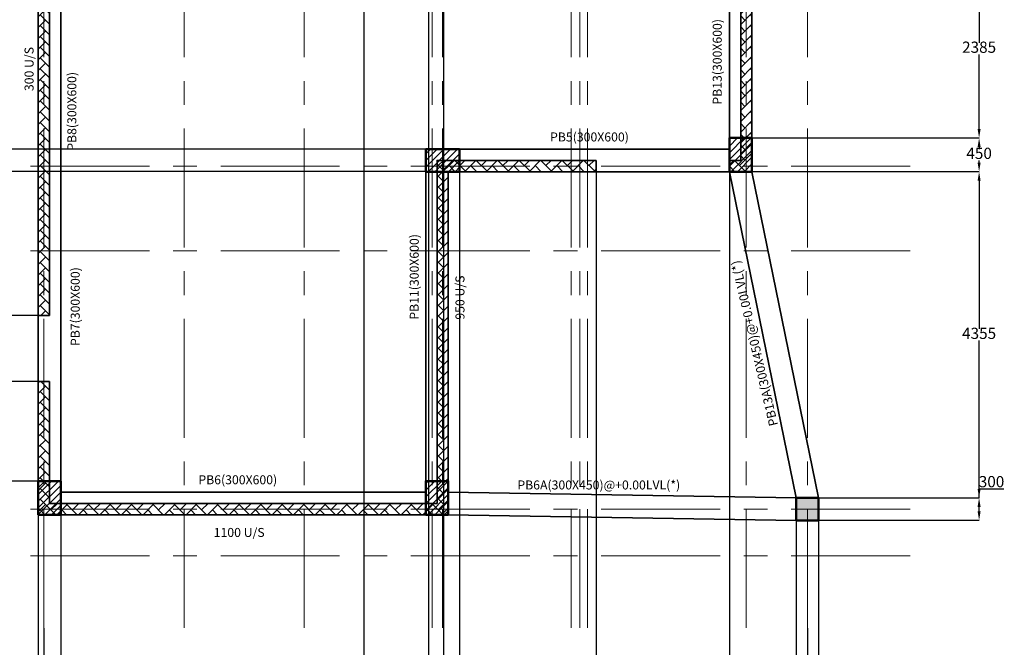
# Model space of a CAD drawing. Units: millimetres. Extents: x -174 to 32373, y 27344 to 53129.
# Tile 4 of 7: x 8204 to 21352, y 36674 to 45053. Entities that reach past the tile are written whole.
import ezdxf

# ---------------------------------------------------------------- set-up
doc = ezdxf.new("R2010")
doc.units = ezdxf.units.MM
doc.header["$LTSCALE"] = 50
doc.linetypes.add('CENTER', pattern=[50.8, 31.75, -6.35, 6.35, -6.35])
for name, color, linetype, lineweight in [('S-ANNO-DIMS', 2, 'Continuous', 18), ('S-ANNO-TEXT', 3, 'Continuous', 18), ('S-BEAM', 7, 'Continuous', 35), ('S-COLS', 1, 'Continuous', 50), ('S-GRID', 8, 'CENTER', 18), ('S-PATT', 8, 'Continuous', 13)]:
    doc.layers.add(name, color=color, linetype=linetype, lineweight=lineweight)
doc.styles.get("Standard").update_dxf_attribs({"font": 'arial.ttf'})
doc.dimstyles.new('ISO-25', dxfattribs={"dimtxt": 150, "dimasz": 120, "dimexe": 1.25, "dimexo": 0.625, "dimtad": 1, "dimtih": 1, "dimtoh": 1, "dimdec": 0, "dimtxsty": 'Standard', "dimcen": 2.5, "dimadec": 0, "dimazin": 0, "dimtfac": 1, "dimtdec": 0, "dimtmove": 0, "dimatfit": 3, "dimfxl": 1, "dimarcsym": 0})

# ---------------------------------------------------------------- blocks, each defined once
blk = doc.blocks.new('*D36')
at = {"layer": 'Defpoints', "color": 0, "transparency": 16777216}
for p in [(8452, 38444), (18872, 38369), (18872, 34336)]:
    blk.add_point(p, dxfattribs=at)
at = {"layer": 'S-ANNO-DIMS', "color": 0, "lineweight": -2, "transparency": 16777216}
for p, q in [((8452, 38443), (8452, 34335)), ((18872, 38368), (18872, 34335)), ((8572, 34336), (18752, 34336))]:
    blk.add_line(p, q, dxfattribs=at)
at = {"layer": 'S-ANNO-DIMS', "color": 0, "transparency": 16777216}
for points in [[(8572, 34356), (8572, 34316), (8452, 34336)], [(18752, 34356), (18752, 34316), (18872, 34336)]]:
    blk.add_solid(points, dxfattribs=at)
at = {"layer": 'S-ANNO-DIMS', "color": 0, "transparency": 16777216, "insert": (13662, 34413), "char_height": 150, "attachment_point": 5}
blk.add_mtext('10420', dxfattribs=at)
blk = doc.blocks.new('*D37')
at = {"layer": 'Defpoints', "color": 0, "transparency": 16777216}
for p in [(8452, 38444), (8527, 36932), (8527, 34336)]:
    blk.add_point(p, dxfattribs=at)
at = {"layer": 'S-ANNO-DIMS', "color": 0, "lineweight": -2, "transparency": 16777216}
for p, q in [((8452, 38443), (8452, 34335)), ((8527, 36931), (8527, 34335)), ((8332, 34336), (8212, 34336)), ((8452, 34336), (8527, 34336)), ((8647, 34336), (8983, 34336))]:
    blk.add_line(p, q, dxfattribs=at)
at = {"layer": 'S-ANNO-DIMS', "color": 0, "transparency": 16777216}
for points in [[(8332, 34356), (8332, 34316), (8452, 34336)], [(8647, 34356), (8647, 34316), (8527, 34336)]]:
    blk.add_solid(points, dxfattribs=at)
at = {"layer": 'S-ANNO-DIMS', "color": 0, "transparency": 16777216, "insert": (8875, 34413), "char_height": 150, "attachment_point": 5}
blk.add_mtext('75', dxfattribs=at)
blk = doc.blocks.new('*D38')
at = {"layer": 'Defpoints', "color": 0, "transparency": 16777216}
for p in [(18572, 38369), (18722, 36932), (18722, 34336)]:
    blk.add_point(p, dxfattribs=at)
at = {"layer": 'S-ANNO-DIMS', "color": 0, "lineweight": -2, "transparency": 16777216}
for p, q in [((18572, 38368), (18572, 34335)), ((18722, 36931), (18722, 34335)), ((18452, 34336), (18332, 34336)), ((18572, 34336), (18722, 34336)), ((18842, 34336), (19280, 34336))]:
    blk.add_line(p, q, dxfattribs=at)
at = {"layer": 'S-ANNO-DIMS', "color": 0, "transparency": 16777216}
for points in [[(18452, 34356), (18452, 34316), (18572, 34336)], [(18842, 34356), (18842, 34316), (18722, 34336)]]:
    blk.add_solid(points, dxfattribs=at)
at = {"layer": 'S-ANNO-DIMS', "color": 0, "transparency": 16777216, "insert": (19121, 34413), "char_height": 150, "attachment_point": 5}
blk.add_mtext('150', dxfattribs=at)
blk = doc.blocks.new('*D41')
at = {"layer": 'Defpoints', "color": 0, "transparency": 16777216}
for p in [(8452, 38444), (8752, 38444), (8752, 34336)]:
    blk.add_point(p, dxfattribs=at)
at = {"layer": 'S-ANNO-DIMS', "color": 0, "lineweight": -2, "transparency": 16777216}
for p, q in [((8452, 38443), (8452, 34335)), ((8752, 38443), (8752, 34335)), ((8572, 34336), (8632, 34336)), ((8752, 34336), (9204, 34336))]:
    blk.add_line(p, q, dxfattribs=at)
at = {"layer": 'S-ANNO-DIMS', "color": 0, "transparency": 16777216}
for points in [[(8572, 34356), (8572, 34316), (8452, 34336)], [(8632, 34356), (8632, 34316), (8752, 34336)]]:
    blk.add_solid(points, dxfattribs=at)
at = {"layer": 'S-ANNO-DIMS', "color": 0, "transparency": 16777216, "insert": (9038, 34413), "char_height": 150, "attachment_point": 5}
blk.add_mtext('300', dxfattribs=at)
blk = doc.blocks.new('*D43')
at = {"layer": 'Defpoints', "color": 0, "transparency": 16777216}
for p in [(1935, 43324), (13627, 43324), (13627, 43024)]:
    blk.add_point(p, dxfattribs=at)
at = {"layer": 'S-ANNO-DIMS', "color": 0, "lineweight": -2, "transparency": 16777216}
for p, q in [((1935, 43324), (1935, 43444)), ((1935, 43444), (2267, 43444)), ((13626, 43324), (1934, 43324)), ((1935, 43144), (1935, 43204)), ((13626, 43024), (1934, 43024))]:
    blk.add_line(p, q, dxfattribs=at)
at = {"layer": 'S-ANNO-DIMS', "color": 0, "transparency": 16777216}
for points in [[(1915, 43204), (1955, 43204), (1935, 43324)], [(1915, 43144), (1955, 43144), (1935, 43024)]]:
    blk.add_solid(points, dxfattribs=at)
at = {"layer": 'S-ANNO-DIMS', "color": 0, "transparency": 16777216, "insert": (2101, 43521), "char_height": 150, "attachment_point": 5}
blk.add_mtext('300', dxfattribs=at)
blk = doc.blocks.new('*D44')
at = {"layer": 'Defpoints', "color": 0, "transparency": 16777216}
for p in [(13662, 45234), (13862, 45234), (13862, 34336)]:
    blk.add_point(p, dxfattribs=at)
at = {"layer": 'S-ANNO-DIMS', "color": 0, "lineweight": -2, "transparency": 16777216}
for p, q in [((13662, 45233), (13662, 34335)), ((13862, 45233), (13862, 34335)), ((13542, 34336), (13422, 34336)), ((13662, 34336), (13862, 34336)), ((13982, 34336), (14436, 34336))]:
    blk.add_line(p, q, dxfattribs=at)
at = {"layer": 'S-ANNO-DIMS', "color": 0, "transparency": 16777216}
for points in [[(13542, 34356), (13542, 34316), (13662, 34336)], [(13982, 34356), (13982, 34316), (13862, 34336)]]:
    blk.add_solid(points, dxfattribs=at)
at = {"layer": 'S-ANNO-DIMS', "color": 0, "transparency": 16777216, "insert": (14269, 34413), "char_height": 150, "attachment_point": 5}
blk.add_mtext('200', dxfattribs=at)
blk = doc.blocks.new('*D46')
at = {"layer": 'Defpoints', "color": 0, "transparency": 16777216}
for p in [(18572, 38369), (18872, 38369), (18872, 34336)]:
    blk.add_point(p, dxfattribs=at)
at = {"layer": 'S-ANNO-DIMS', "color": 0, "lineweight": -2, "transparency": 16777216}
for p, q in [((18572, 38368), (18572, 34335)), ((18872, 38368), (18872, 34335)), ((18692, 34336), (18752, 34336)), ((18872, 34336), (19324, 34336))]:
    blk.add_line(p, q, dxfattribs=at)
at = {"layer": 'S-ANNO-DIMS', "color": 0, "transparency": 16777216}
for points in [[(18692, 34356), (18692, 34316), (18572, 34336)], [(18752, 34356), (18752, 34316), (18872, 34336)]]:
    blk.add_solid(points, dxfattribs=at)
at = {"layer": 'S-ANNO-DIMS', "color": 0, "transparency": 16777216, "insert": (19158, 34413), "char_height": 150, "attachment_point": 5}
blk.add_mtext('300', dxfattribs=at)
blk = doc.blocks.new('*D47')
at = {"layer": 'Defpoints', "color": 0, "transparency": 16777216}
for p in [(18872, 38669), (21015, 38669), (18872, 38369)]:
    blk.add_point(p, dxfattribs=at)
at = {"layer": 'S-ANNO-DIMS', "color": 0, "lineweight": -2, "transparency": 16777216}
for p, q in [((21015, 38669), (21015, 38789)), ((21015, 38789), (21347, 38789)), ((18872, 38669), (21016, 38669)), ((21015, 38489), (21015, 38549)), ((18872, 38369), (21016, 38369))]:
    blk.add_line(p, q, dxfattribs=at)
at = {"layer": 'S-ANNO-DIMS', "color": 0, "transparency": 16777216}
for points in [[(20995, 38549), (21035, 38549), (21015, 38669)], [(20995, 38489), (21035, 38489), (21015, 38369)]]:
    blk.add_solid(points, dxfattribs=at)
at = {"layer": 'S-ANNO-DIMS', "color": 0, "transparency": 16777216, "insert": (21181, 38866), "char_height": 150, "attachment_point": 5}
blk.add_mtext('300', dxfattribs=at)
blk = doc.blocks.new('*D48')
at = {"layer": 'Defpoints', "color": 0, "transparency": 16777216}
for p in [(17682, 43024), (18572, 38669), (18572, 34336)]:
    blk.add_point(p, dxfattribs=at)
at = {"layer": 'S-ANNO-DIMS', "color": 0, "lineweight": -2, "transparency": 16777216}
for p, q in [((17682, 43023), (17682, 34335)), ((18572, 38668), (18572, 34335)), ((17802, 34336), (18452, 34336))]:
    blk.add_line(p, q, dxfattribs=at)
at = {"layer": 'S-ANNO-DIMS', "color": 0, "transparency": 16777216}
for points in [[(17802, 34356), (17802, 34316), (17682, 34336)], [(18452, 34356), (18452, 34316), (18572, 34336)]]:
    blk.add_solid(points, dxfattribs=at)
at = {"layer": 'S-ANNO-DIMS', "color": 0, "transparency": 16777216, "insert": (18127, 34413), "char_height": 150, "attachment_point": 5}
blk.add_mtext('890', dxfattribs=at)
blk = doc.blocks.new('*D49')
at = {"layer": 'Defpoints', "color": 0, "transparency": 16777216}
for p in [(17982, 43024), (18872, 38669), (21015, 38669)]:
    blk.add_point(p, dxfattribs=at)
at = {"layer": 'S-ANNO-DIMS', "color": 0, "lineweight": -2, "transparency": 16777216}
for p, q in [((17982, 43024), (21016, 43024)), ((21015, 42904), (21015, 40924)), ((21015, 38789), (21015, 40769)), ((18872, 38669), (21016, 38669))]:
    blk.add_line(p, q, dxfattribs=at)
at = {"layer": 'S-ANNO-DIMS', "color": 0, "transparency": 16777216}
for points in [[(20995, 42904), (21035, 42904), (21015, 43024)], [(20995, 38789), (21035, 38789), (21015, 38669)]]:
    blk.add_solid(points, dxfattribs=at)
at = {"layer": 'S-ANNO-DIMS', "color": 0, "transparency": 16777216, "insert": (21015, 40846), "char_height": 150, "attachment_point": 5}
blk.add_mtext('4355', dxfattribs=at)
blk = doc.blocks.new('*D52')
at = {"layer": 'Defpoints', "color": 0, "transparency": 16777216}
for p in [(17982, 45859), (17982, 43474), (21015, 43474)]:
    blk.add_point(p, dxfattribs=at)
at = {"layer": 'S-ANNO-DIMS', "color": 0, "lineweight": -2, "transparency": 16777216}
for p, q in [((17982, 45859), (21016, 45859)), ((21015, 45739), (21015, 44744)), ((21015, 43594), (21015, 44589)), ((17982, 43474), (21016, 43474))]:
    blk.add_line(p, q, dxfattribs=at)
at = {"layer": 'S-ANNO-DIMS', "color": 0, "transparency": 16777216}
for points in [[(20995, 45739), (21035, 45739), (21015, 45859)], [(20995, 43594), (21035, 43594), (21015, 43474)]]:
    blk.add_solid(points, dxfattribs=at)
at = {"layer": 'S-ANNO-DIMS', "color": 0, "transparency": 16777216, "insert": (21015, 44666), "char_height": 150, "attachment_point": 5}
blk.add_mtext('2385', dxfattribs=at)
blk = doc.blocks.new('*D53')
at = {"layer": 'Defpoints', "color": 0, "transparency": 16777216}
for p in [(17982, 43474), (17982, 43024), (21015, 43024)]:
    blk.add_point(p, dxfattribs=at)
at = {"layer": 'S-ANNO-DIMS', "color": 0, "lineweight": -2, "transparency": 16777216}
for p, q in [((17982, 43474), (21016, 43474)), ((21015, 43354), (21015, 43326)), ((21015, 43144), (21015, 43172)), ((17982, 43024), (21016, 43024))]:
    blk.add_line(p, q, dxfattribs=at)
at = {"layer": 'S-ANNO-DIMS', "color": 0, "transparency": 16777216}
for points in [[(20995, 43354), (21035, 43354), (21015, 43474)], [(20995, 43144), (21035, 43144), (21015, 43024)]]:
    blk.add_solid(points, dxfattribs=at)
at = {"layer": 'S-ANNO-DIMS', "color": 0, "transparency": 16777216, "insert": (21015, 43249), "char_height": 150, "attachment_point": 5}
blk.add_mtext('450', dxfattribs=at)
blk = doc.blocks.new('*D56')
at = {"layer": 'Defpoints', "color": 0, "transparency": 16777216}
for p in [(1935, 40221), (8452, 40221), (8452, 38894)]:
    blk.add_point(p, dxfattribs=at)
at = {"layer": 'S-ANNO-DIMS', "color": 0, "lineweight": -2, "transparency": 16777216}
for p, q in [((8451, 40221), (1934, 40221)), ((1935, 40101), (1935, 39635)), ((1935, 39014), (1935, 39480)), ((8451, 38894), (1934, 38894))]:
    blk.add_line(p, q, dxfattribs=at)
at = {"layer": 'S-ANNO-DIMS', "color": 0, "transparency": 16777216}
for points in [[(1915, 40101), (1955, 40101), (1935, 40221)], [(1915, 39014), (1955, 39014), (1935, 38894)]]:
    blk.add_solid(points, dxfattribs=at)
at = {"layer": 'S-ANNO-DIMS', "color": 0, "transparency": 16777216, "insert": (1935, 39557), "char_height": 150, "attachment_point": 5}
blk.add_mtext('1327.4', dxfattribs=at)
blk = doc.blocks.new('*D57')
at = {"layer": 'Defpoints', "color": 0, "transparency": 16777216}
for p in [(1935, 41103), (8452, 41103), (8452, 40221)]:
    blk.add_point(p, dxfattribs=at)
at = {"layer": 'S-ANNO-DIMS', "color": 0, "lineweight": -2, "transparency": 16777216}
for p, q in [((8451, 41103), (1934, 41103)), ((1935, 40983), (1935, 40739)), ((1935, 40341), (1935, 40585)), ((8451, 40221), (1934, 40221))]:
    blk.add_line(p, q, dxfattribs=at)
at = {"layer": 'S-ANNO-DIMS', "color": 0, "transparency": 16777216}
for points in [[(1915, 40983), (1955, 40983), (1935, 41103)], [(1915, 40341), (1955, 40341), (1935, 40221)]]:
    blk.add_solid(points, dxfattribs=at)
at = {"layer": 'S-ANNO-DIMS', "color": 0, "transparency": 16777216, "insert": (1935, 40662), "char_height": 150, "attachment_point": 5}
blk.add_mtext('882.1', dxfattribs=at)
blk = doc.blocks.new('*D58')
at = {"layer": 'Defpoints', "color": 0, "transparency": 16777216}
for p in [(15900, 43174), (14077, 43024), (14077, 34336)]:
    blk.add_point(p, dxfattribs=at)
at = {"layer": 'S-ANNO-DIMS', "color": 0, "lineweight": -2, "transparency": 16777216}
for p, q in [((15900, 43173), (15900, 34335)), ((14077, 43023), (14077, 34335)), ((15780, 34336), (14197, 34336))]:
    blk.add_line(p, q, dxfattribs=at)
at = {"layer": 'S-ANNO-DIMS', "color": 0, "transparency": 16777216}
for points in [[(14197, 34356), (14197, 34316), (14077, 34336)], [(15780, 34356), (15780, 34316), (15900, 34336)]]:
    blk.add_solid(points, dxfattribs=at)
at = {"layer": 'S-ANNO-DIMS', "color": 0, "transparency": 16777216, "insert": (14988, 34413), "char_height": 150, "attachment_point": 5}
blk.add_mtext('1823', dxfattribs=at)
blk = doc.blocks.new('*D59')
at = {"layer": 'Defpoints', "color": 0, "transparency": 16777216}
for p in [(12800, 46609), (13662, 46609), (13662, 34336)]:
    blk.add_point(p, dxfattribs=at)
at = {"layer": 'S-ANNO-DIMS', "color": 0, "lineweight": -2, "transparency": 16777216}
for p, q in [((12800, 46608), (12800, 34335)), ((13662, 46608), (13662, 34335)), ((12920, 34336), (13542, 34336))]:
    blk.add_line(p, q, dxfattribs=at)
at = {"layer": 'S-ANNO-DIMS', "color": 0, "transparency": 16777216}
for points in [[(12920, 34356), (12920, 34316), (12800, 34336)], [(13542, 34356), (13542, 34316), (13662, 34336)]]:
    blk.add_solid(points, dxfattribs=at)
at = {"layer": 'S-ANNO-DIMS', "color": 0, "transparency": 16777216, "insert": (13231, 34413), "char_height": 150, "attachment_point": 5}
blk.add_mtext('862', dxfattribs=at)

msp = doc.modelspace()

# ---------------------------------------------------------------- hatches: boundary and pattern name
at = {"layer": 'S-PATT'}
h = msp.add_hatch(dxfattribs=at)
h.set_pattern_fill('AR-HBONE', color=256)
h.paths.add_polyline_path([(8601.66, 48993.76), (14749, 48993.76), (14749, 49143.76), (8451.66, 49143.76), (8451.66, 41103.32), (8601.66, 41103.32)])
h = msp.add_hatch(dxfattribs=at)
h.set_pattern_fill('AR-HBONE', color=256)
h.paths.add_polyline_path([(17981.66, 49143.76), (16815.46, 49143.76), (16815.46, 48993.76), (17831.66, 48993.76), (17831.66, 43173.76), (17681.66, 43173.76), (17681.66, 43023.76), (17981.66, 43023.76)])
h = msp.add_hatch(dxfattribs=at)
h.set_pattern_fill('ANSI31', color=256, scale=20)
h.paths.add_polyline_path([(17981.66, 43473.76), (17681.66, 43473.76), (17681.66, 43023.76), (17981.66, 43023.76)])
h = msp.add_hatch(dxfattribs=at)
h.set_pattern_fill('ANSI31', color=256, scale=20)
h.paths.add_polyline_path([(14076.66, 43323.76), (13626.66, 43323.76), (13626.66, 43023.76), (14076.66, 43023.76)])
h = msp.add_hatch(dxfattribs=at)
h.set_pattern_fill('AR-HBONE', color=256)
h.paths.add_polyline_path([(15899.72, 43173.76), (13776.66, 43173.76), (13776.66, 38593.76), (8601.66, 38593.76), (8601.66, 40221.18), (8451.66, 40221.18), (8451.66, 38443.76), (13926.66, 38443.76), (13926.66, 43023.76), (15899.72, 43023.76)])
h = msp.add_hatch(dxfattribs=at)
h.set_pattern_fill('ANSI31', color=256, scale=20)
h.paths.add_polyline_path([(8751.66, 38893.76), (8451.66, 38893.76), (8451.66, 38443.76), (8751.66, 38443.76)])
h = msp.add_hatch(dxfattribs=at)
h.set_pattern_fill('ANSI31', color=256, scale=20)
h.paths.add_polyline_path([(13926.66, 38893.76), (13626.66, 38893.76), (13626.66, 38443.76), (13926.66, 38443.76)])
h = msp.add_hatch(color=256, dxfattribs=at)
h.dxf.hatch_style = 1
h.paths.add_polyline_path([(18871.66, 38668.76), (18571.66, 38668.76), (18571.66, 38368.76), (18871.66, 38368.76)])

# ---------------------------------------------------------------- linework, layer by layer
at = {"layer": 'S-BEAM'}
for p, q in [((8451.66, 38443.76), (8451.66, 49143.76)), ((17981.66, 43023.76), (17981.66, 49143.76)), ((17831.66, 43173.76), (17831.66, 48993.76)), ((17681.66, 43323.76), (17681.66, 48843.76)), ((8751.66, 38743.76), (8751.66, 45233.76)), ((13626.66, 38743.76), (13626.66, 43323.76)), ((13626.66, 43323.76), (17681.66, 43323.76)), ((15899.72, 43173.76), (15899.72, 43023.76)), ((17681.66, 43173.76), (17681.66, 43023.76)), ((17981.66, 43023.76), (13926.66, 43023.76)), ((17681.66, 43023.76), (18571.66, 38668.76)), ((17981.66, 43023.76), (18871.66, 38668.76)), ((8601.66, 41103.32), (8451.66, 41103.32)), ((8601.66, 40221.18), (8451.66, 40221.18)), ((13626.66, 38743.76), (8751.66, 38743.76)), ((18571.66, 38668.76), (13926.66, 38743.76)), ((13926.66, 38443.76), (8451.66, 38443.76)), ((13926.66, 38443.76), (18571.66, 38368.76))]:
    msp.add_line(p, q, dxfattribs=at)
for points in [[(8601.66, 48993.76), (8601.66, 41103.32)], [(8601.66, 40221.18), (8601.66, 38593.76), (13776.66, 38593.76), (13776.66, 43173.76), (15899.72, 43173.76)], [(17681.66, 43173.76), (17831.66, 43173.76)], [(13926.66, 38443.76), (13926.66, 43023.76)]]:
    msp.add_lwpolyline(points, dxfattribs=at)
at = {"layer": 'S-COLS'}
for points in [[(17681.66, 43023.76), (17981.66, 43023.76), (17981.66, 43473.76), (17681.66, 43473.76)], [(13626.66, 43323.76), (13626.66, 43023.76), (14076.66, 43023.76), (14076.66, 43323.76)], [(8451.66, 38443.76), (8751.66, 38443.76), (8751.66, 38893.76), (8451.66, 38893.76)], [(13626.66, 38443.76), (13926.66, 38443.76), (13926.66, 38893.76), (13626.66, 38893.76)], [(18871.66, 38668.76), (18571.66, 38668.76), (18571.66, 38368.76), (18871.66, 38368.76)]]:
    msp.add_lwpolyline(points, close=True, dxfattribs=at)
at = {"layer": 'S-GRID'}
for p, q in [((8526.66, 36931.64), (8526.66, 51397.21)), ((10401.66, 36931.64), (10401.66, 51397.21)), ((12001.66, 36931.64), (12001.66, 51397.21)), ((15681.66, 36931.64), (15681.66, 51397.21)), ((17906.66, 36931.64), (17906.66, 51397.21)), ((18721.66, 36931.64), (18721.66, 51397.21)), ((20095.15, 43098.76), (3491.75, 43098.76)), ((20095.15, 41968.76), (3491.75, 41968.76)), ((20095.15, 38518.76), (3491.75, 38518.76)), ((20095.15, 37893.76), (3491.75, 37893.76))]:
    msp.add_line(p, q, dxfattribs=at)
for points in [[(13711.66, 36931.64), (13711.66, 50814.23), (13439.61, 51397.21)], [(13851.66, 36931.64), (13851.66, 50814.23), (14122.87, 51397.21)], [(15566.66, 36931.64), (15566.66, 50814.23), (14989.62, 51397.21)], [(15786.66, 36931.64), (15786.66, 50814.23), (16397.9, 51397.21)]]:
    msp.add_lwpolyline(points, dxfattribs=at)

# ---------------------------------------------------------------- texts
at = {"layer": 'S-ANNO-TEXT', "char_height": 120, "attachment_point": 1}
for s, insert, rotation in [('PB13(300X600)', (17458.5, 43919.04), 90), ('300 U/S', (8269.3, 44099.59), 90), ('PB8(300X600)', (8840.23, 43303.19), 90), ('PB11(300X600)', (13412.27, 41047.92), 90), ('PB13A(300X450)@+0.00LVL(*)', (18214.13, 39615.75), 103.101328), ('PB7(300X600)', (8885.53, 40696.4), 90), ('950 U/S', (14022.81, 41047.92), 90)]:
    msp.add_mtext_dynamic_manual_height_columns(s, width=1913.0414, gutter_width=12.5, heights=[0], dxfattribs=dict(at, insert=insert, rotation=rotation))
for s, insert in [('PB5(300X600)', (15286.35, 43547.07)), ('PB6(300X600)', (10590.25, 38970.34)), ('PB6A(300X450)@+0.00LVL(*)', (14849.79, 38901.13)), ('1100 U/S', (10794.81, 38267.06))]:
    msp.add_mtext_dynamic_manual_height_columns(s, width=1913.0414, gutter_width=12.5, heights=[0], dxfattribs=dict(at, insert=insert))

# ---------------------------------------------------------------- dimensions: what is measured, and where the dimension line sits
at = {"layer": 'S-ANNO-DIMS'}
for base, p1, p2, picture, middle in [((13661.66, 34335.75), (12799.66, 46608.76), (13661.66, 46608.76), '*D59', (13230.66, 34412.96)), ((13861.66, 34335.75), (13661.66, 45233.76), (13861.66, 45233.76), '*D44', (14269.02, 34412.96)), ((14076.66, 34335.75), (15899.72, 43173.76), (14076.66, 43023.76), '*D58', (14988.19, 34413.01)), ((18571.66, 34335.75), (17681.66, 43023.76), (18571.66, 38668.76), '*D48', (18126.66, 34412.96)), ((8526.66, 34335.75), (8451.66, 38443.76), (8526.66, 36931.64), '*D37', (8874.67, 34412.65)), ((18871.66, 34335.75), (8451.66, 38443.76), (18871.66, 38368.76), '*D36', (13661.66, 34412.96)), ((8751.66, 34335.75), (8451.66, 38443.76), (8751.66, 38443.76), '*D41', (9037.69, 34413.01)), ((18721.66, 34335.75), (18571.66, 38368.76), (18721.66, 36931.64), '*D38', (19120.68, 34412.96)), ((18871.66, 34335.75), (18571.66, 38368.76), (18871.66, 38368.76), '*D46', (19157.69, 34413.01))]:
    dim = msp.add_linear_dim(base=base, p1=p1, p2=p2, dimstyle='ISO-25', override={"dimdec": 0, "dimlfac": 1, "dimrnd": 0, "dimzin": 0, "dimdsep": 46, "dimlunit": 2}, dxfattribs=at)
    dim.commit()
    dim.dimension.update_dxf_attribs({"geometry": picture, "text_midpoint": middle})
for base, p1, p2, override, picture, middle in [((21015.15, 43473.76), (17981.66, 45858.76), (17981.66, 43473.76), {"dimdec": 0, "dimlfac": 1, "dimrnd": 0, "dimzin": 0, "dimdsep": 46, "dimlunit": 2}, '*D52', (21015.15, 44666.26)), ((1935.38, 43323.76), (13626.66, 43023.76), (13626.66, 43323.76), {"dimdec": 0, "dimlfac": 1, "dimrnd": 0, "dimzin": 0, "dimdsep": 46, "dimlunit": 2}, '*D43', (2101.4, 43521.02)), ((21015.15, 43023.76), (17981.66, 43473.76), (17981.66, 43023.76), {"dimdec": 0, "dimlfac": 1, "dimrnd": 0, "dimzin": 0, "dimdsep": 46, "dimlunit": 2}, '*D53', (21015.15, 43248.76)), ((21015.15, 38668.76), (17981.66, 43023.76), (18871.66, 38668.76), {"dimdec": 0, "dimlfac": 1, "dimrnd": 0, "dimzin": 0, "dimdsep": 46, "dimlunit": 2}, '*D49', (21015.15, 40846.26)), ((1935.38, 41103.32), (8451.66, 40221.18), (8451.66, 41103.32), {"dimdec": 1, "dimlfac": 1, "dimrnd": 0, "dimzin": 0, "dimdsep": 46, "dimlunit": 2}, '*D57', (1935.38, 40662.25)), ((1935.38, 40221.18), (8451.66, 38893.76), (8451.66, 40221.18), {"dimdec": 1, "dimlfac": 1, "dimrnd": 0, "dimzin": 0, "dimdsep": 46, "dimlunit": 2}, '*D56', (1935.38, 39557.47)), ((21015.15, 38668.76), (18871.66, 38368.76), (18871.66, 38668.76), {"dimdec": 0, "dimlfac": 1, "dimrnd": 0, "dimzin": 0, "dimdsep": 46, "dimlunit": 2}, '*D47', (21181.18, 38866.02))]:
    dim = msp.add_linear_dim(base=base, p1=p1, p2=p2, angle=90, dimstyle='ISO-25', override=override, dxfattribs=at)
    dim.commit()
    dim.dimension.update_dxf_attribs({"geometry": picture, "text_midpoint": middle})

doc.saveas('drawing.dxf')
